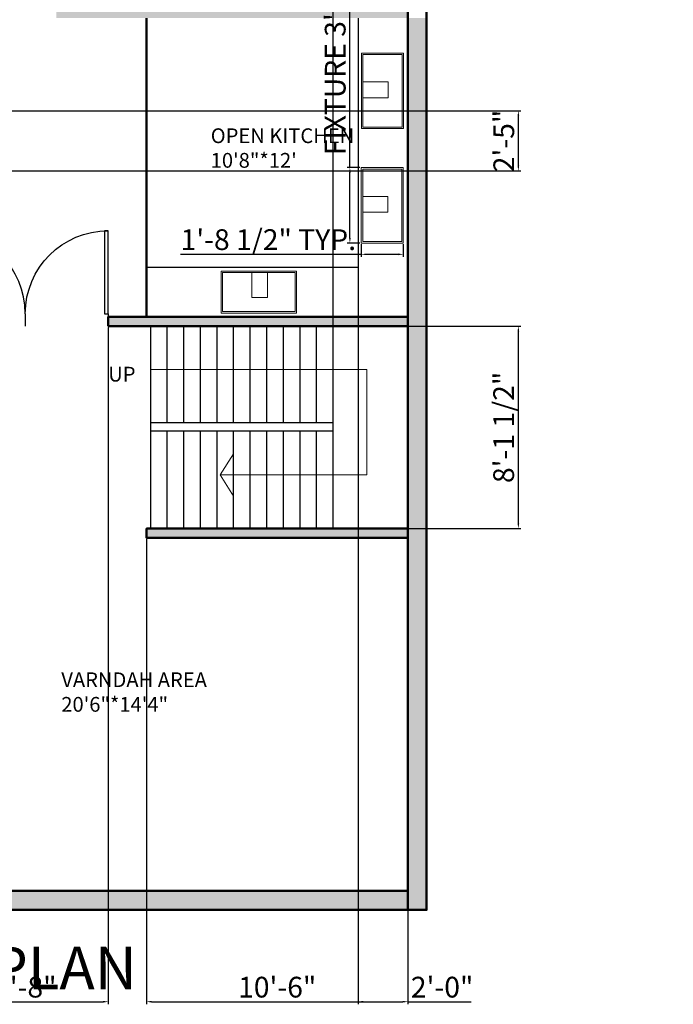
# Model space of a CAD drawing. Units: inches. Extents: x 1477 to 2233, y 1388 to 2326.
# Tile 2 of 4: x 1917 to 2233, y 1396 to 1870. Entities that reach past the tile are written whole.
import ezdxf

# ---------------------------------------------------------------- set-up
doc = ezdxf.new("R2010")
doc.units = ezdxf.units.IN
for name, color, linetype, lineweight in [('A-ANNO-DIMS', 2, 'Continuous', 18), ('A-ANNO-SYMB', 7, 'Continuous', 18), ('A-ANNO-TEXT', 7, 'Continuous', 35), ('A-AREA-IDEN', 7, 'Continuous', 18), ('A-DOOR', 4, 'Continuous', 25), ('A-FLOR-CASE', 9, 'Continuous', 25), ('A-FLOR-FIXT', 8, 'Continuous', 18), ('A-FLOR-STRS', 7, 'Continuous', 25), ('A-WALL-PATT', 10, 'Continuous', 13), ('wall', 10, 'Continuous', 50)]:
    doc.layers.add(name, color=color, linetype=linetype, lineweight=lineweight)
doc.styles.get("Standard").update_dxf_attribs({"font": 'arial.ttf'})
doc.dimstyles.new('ISO-25', dxfattribs={"dimtxt": 10, "dimasz": 2.5, "dimexe": 1.25, "dimexo": 0.625, "dimtad": 1, "dimdec": 0, "dimlunit": 4, "dimtxsty": 'Standard', "dimcen": 2.5, "dimadec": 0, "dimazin": 0, "dimtfac": 1, "dimtdec": 0, "dimtmove": 0, "dimatfit": 3, "dimfxl": 1, "dimarcsym": 0})

# ---------------------------------------------------------------- blocks, each defined once
blk = doc.blocks.new('*U2')
for p, q in [((0, 0), (0, -6)), ((40, 0), (40, -6))]:
    blk.add_line(p, q)
blk.add_lwpolyline([(0, 0), (0, 40), (1.75, 40), (1.75, 0)], close=True)
blk.add_arc((0, 0), 40, 0, 90)
blk = doc.blocks.new('KITCHEN-FIXTURE')
for points in [[(0, 20.26), (36.38, 20.26), (36.38, 0), (0, 0)], [(0.72, 19.54), (35.67, 19.54), (35.67, 0.72), (0.72, 0.72)], [(14.83, 19.54), (22.43, 19.54), (22.43, 7.46), (14.83, 7.46)]]:
    blk.add_lwpolyline(points, close=True)
blk = doc.blocks.new('*D25')
at = {"layer": 'A-ANNO-DIMS', "color": 0, "lineweight": -2, "transparency": 16777216}
for p, q in [((2033, 1898.51), (2033, 1887.14)), ((2104.61, 1898.51), (2104.61, 1887.14)), ((2035.5, 1888.39), (2102.11, 1888.39)), ((2104.61, 1888.39), (2232.55, 1888.39))]:
    blk.add_line(p, q, dxfattribs=at)
at = {"layer": 'A-ANNO-DIMS', "color": 0, "transparency": 16777216}
for points in [[(2035.5, 1888.81), (2035.5, 1887.97), (2033, 1888.39)], [(2102.11, 1888.81), (2102.11, 1887.97), (2104.61, 1888.39)]]:
    blk.add_solid(points, dxfattribs=at)
at = {"layer": 'Defpoints', "color": 0, "transparency": 16777216}
for p in [(2033, 1899.13), (2104.61, 1899.13), (2104.61, 1888.39)]:
    blk.add_point(p, dxfattribs=at)
at = {"layer": 'A-ANNO-DIMS', "color": 0, "transparency": 16777216, "insert": (2169.83, 1894.18), "char_height": 10, "attachment_point": 5}
blk.add_mtext('BED 5\'-11 1/2" TYP.', dxfattribs=at)
blk = doc.blocks.new('*D29')
at = {"layer": 'A-ANNO-DIMS', "color": 0, "lineweight": -2, "transparency": 16777216}
for p, q in [((2076.64, 1799.12), (2076.64, 1950.21)), ((2081.48, 1799.12), (2075.39, 1799.12)), ((2076.64, 1765.24), (2076.64, 1796.62)), ((2081.48, 1762.74), (2075.39, 1762.74))]:
    blk.add_line(p, q, dxfattribs=at)
at = {"layer": 'A-ANNO-DIMS', "color": 0, "transparency": 16777216}
for points in [[(2076.23, 1796.62), (2077.06, 1796.62), (2076.64, 1799.12)], [(2076.23, 1765.24), (2077.06, 1765.24), (2076.64, 1762.74)]]:
    blk.add_solid(points, dxfattribs=at)
at = {"layer": 'Defpoints', "color": 0, "transparency": 16777216}
for p in [(2076.64, 1799.12), (2082.1, 1799.12), (2082.1, 1762.74)]:
    blk.add_point(p, dxfattribs=at)
at = {"layer": 'A-ANNO-DIMS', "color": 0, "transparency": 16777216, "insert": (2070.85, 1875.92), "char_height": 10, "attachment_point": 5, "rotation": 90}
blk.add_mtext('FIXTURE 3\'-0 1/2" TYP.', dxfattribs=at)
blk = doc.blocks.new('*D30')
at = {"layer": 'A-ANNO-DIMS', "color": 0, "lineweight": -2, "transparency": 16777216}
for p, q in [((2082.1, 1762.11), (2082.1, 1756.03)), ((2102.36, 1762.11), (2102.36, 1756.03)), ((2082.1, 1757.28), (1995.04, 1757.28)), ((2099.86, 1757.28), (2084.6, 1757.28))]:
    blk.add_line(p, q, dxfattribs=at)
at = {"layer": 'A-ANNO-DIMS', "color": 0, "transparency": 16777216}
for points in [[(2084.6, 1757.7), (2084.6, 1756.87), (2082.1, 1757.28)], [(2099.86, 1757.7), (2099.86, 1756.87), (2102.36, 1757.28)]]:
    blk.add_solid(points, dxfattribs=at)
at = {"layer": 'Defpoints', "color": 0, "transparency": 16777216}
for p in [(2082.1, 1762.74), (2102.36, 1762.74), (2082.1, 1757.28)]:
    blk.add_point(p, dxfattribs=at)
at = {"layer": 'A-ANNO-DIMS', "color": 0, "transparency": 16777216, "insert": (2037.32, 1763.08), "char_height": 10, "attachment_point": 5}
blk.add_mtext('1\'-8 1/2" TYP.', dxfattribs=at)
blk = doc.blocks.new('*D33')
at = {"layer": 'A-ANNO-DIMS', "color": 0, "lineweight": -2, "transparency": 16777216}
for p, q in [((1880.17, 1722.05), (1880.17, 1395.67)), ((1960.17, 1722.05), (1960.17, 1395.67)), ((1882.67, 1396.92), (1957.67, 1396.92))]:
    blk.add_line(p, q, dxfattribs=at)
at = {"layer": 'A-ANNO-DIMS', "color": 0, "transparency": 16777216}
for points in [[(1882.67, 1397.34), (1882.67, 1396.51), (1880.17, 1396.92)], [(1957.67, 1397.34), (1957.67, 1396.51), (1960.17, 1396.92)]]:
    blk.add_solid(points, dxfattribs=at)
at = {"layer": 'Defpoints', "color": 0, "transparency": 16777216}
for p in [(1880.17, 1722.67), (1960.17, 1722.67), (1960.17, 1396.92)]:
    blk.add_point(p, dxfattribs=at)
at = {"layer": 'A-ANNO-DIMS', "color": 0, "transparency": 16777216, "insert": (1920.17, 1402.65), "char_height": 10, "attachment_point": 5}
blk.add_mtext('6\'-8"', dxfattribs=at)
blk = doc.blocks.new('*D34')
at = {"layer": 'A-ANNO-DIMS', "color": 0, "lineweight": -2, "transparency": 16777216}
for p, q in [((1978.61, 1619.91), (1978.61, 1395.67)), ((2104.61, 1619.91), (2104.61, 1395.67)), ((1981.11, 1396.92), (2102.11, 1396.92))]:
    blk.add_line(p, q, dxfattribs=at)
at = {"layer": 'A-ANNO-DIMS', "color": 0, "transparency": 16777216}
for points in [[(1981.11, 1397.34), (1981.11, 1396.51), (1978.61, 1396.92)], [(2102.11, 1397.34), (2102.11, 1396.51), (2104.61, 1396.92)]]:
    blk.add_solid(points, dxfattribs=at)
at = {"layer": 'Defpoints', "color": 0, "transparency": 16777216}
for p in [(1978.61, 1620.53), (2104.61, 1620.53), (2104.61, 1396.92)]:
    blk.add_point(p, dxfattribs=at)
at = {"layer": 'A-ANNO-DIMS', "color": 0, "transparency": 16777216, "insert": (2041.61, 1402.65), "char_height": 10, "attachment_point": 5}
blk.add_mtext('10\'-6"', dxfattribs=at)
blk = doc.blocks.new('*D35')
at = {"layer": 'A-ANNO-DIMS', "color": 0, "lineweight": -2, "transparency": 16777216}
for p, q in [((2068.61, 1625.95), (2068.61, 2252.67)), ((2071.11, 2251.42), (2102.11, 2251.42)), ((2104.61, 1625.66), (2104.61, 2252.67))]:
    blk.add_line(p, q, dxfattribs=at)
at = {"layer": 'A-ANNO-DIMS', "color": 0, "transparency": 16777216}
for points in [[(2071.11, 2251.84), (2071.11, 2251.01), (2068.61, 2251.42)], [(2102.11, 2251.84), (2102.11, 2251.01), (2104.61, 2251.42)]]:
    blk.add_solid(points, dxfattribs=at)
at = {"layer": 'Defpoints', "color": 0, "transparency": 16777216}
for p in [(2104.61, 2251.42), (2068.61, 1625.33), (2104.61, 1625.03)]:
    blk.add_point(p, dxfattribs=at)
at = {"layer": 'A-ANNO-DIMS', "color": 0, "transparency": 16777216, "insert": (2086.61, 2257.16), "char_height": 10, "attachment_point": 5}
blk.add_mtext('3\'-0"', dxfattribs=at)
blk = doc.blocks.new('*D36')
at = {"layer": 'A-ANNO-DIMS', "color": 0, "lineweight": -2, "transparency": 16777216}
for p, q in [((2105.23, 1722.67), (2159.11, 1722.67)), ((2157.86, 1627.53), (2157.86, 1720.17)), ((2105.23, 1625.03), (2159.11, 1625.03))]:
    blk.add_line(p, q, dxfattribs=at)
at = {"layer": 'A-ANNO-DIMS', "color": 0, "transparency": 16777216}
for points in [[(2157.44, 1720.17), (2158.27, 1720.17), (2157.86, 1722.67)], [(2157.44, 1627.53), (2158.27, 1627.53), (2157.86, 1625.03)]]:
    blk.add_solid(points, dxfattribs=at)
at = {"layer": 'Defpoints', "color": 0, "transparency": 16777216}
for p in [(2104.61, 1722.67), (2157.86, 1722.67), (2104.61, 1625.03)]:
    blk.add_point(p, dxfattribs=at)
at = {"layer": 'A-ANNO-DIMS', "color": 0, "transparency": 16777216, "insert": (2152.06, 1673.85), "char_height": 10, "attachment_point": 5, "rotation": 90}
blk.add_mtext('8\'-1 1/2"', dxfattribs=at)
blk = doc.blocks.new('*D37')
at = {"layer": 'A-ANNO-DIMS', "color": 0, "lineweight": -2, "transparency": 16777216}
for p, q in [((2080.61, 1870.55), (2080.61, 1395.67)), ((2104.61, 1870.55), (2104.61, 1395.67)), ((2083.11, 1396.92), (2102.11, 1396.92)), ((2104.61, 1396.92), (2135.11, 1396.92))]:
    blk.add_line(p, q, dxfattribs=at)
at = {"layer": 'A-ANNO-DIMS', "color": 0, "transparency": 16777216}
for points in [[(2083.11, 1397.34), (2083.11, 1396.51), (2080.61, 1396.92)], [(2102.11, 1397.34), (2102.11, 1396.51), (2104.61, 1396.92)]]:
    blk.add_solid(points, dxfattribs=at)
at = {"layer": 'Defpoints', "color": 0, "transparency": 16777216}
for p in [(2080.61, 1871.17), (2104.61, 1871.17), (2104.61, 1396.92)]:
    blk.add_point(p, dxfattribs=at)
at = {"layer": 'A-ANNO-DIMS', "color": 0, "transparency": 16777216, "insert": (2121.11, 1402.65), "char_height": 10, "attachment_point": 5}
blk.add_mtext('2\'-0"', dxfattribs=at)
blk = doc.blocks.new('*D44')
at = {"layer": 'A-ANNO-DIMS', "color": 0, "lineweight": -2, "transparency": 16777216}
for p, q in [((1855.11, 1826.44), (2159.11, 1826.44)), ((2157.86, 1799.98), (2157.86, 1823.94)), ((1855.35, 1797.48), (2159.11, 1797.48))]:
    blk.add_line(p, q, dxfattribs=at)
at = {"layer": 'A-ANNO-DIMS', "color": 0, "transparency": 16777216}
for points in [[(2157.44, 1823.94), (2158.27, 1823.94), (2157.86, 1826.44)], [(2157.44, 1799.98), (2158.27, 1799.98), (2157.86, 1797.48)]]:
    blk.add_solid(points, dxfattribs=at)
at = {"layer": 'Defpoints', "color": 0, "transparency": 16777216}
for p in [(1854.49, 1826.44), (2157.86, 1826.44), (1854.73, 1797.48)]:
    blk.add_point(p, dxfattribs=at)
at = {"layer": 'A-ANNO-DIMS', "color": 0, "transparency": 16777216, "insert": (2152.13, 1811.96), "char_height": 10, "attachment_point": 5, "rotation": 90}
blk.add_mtext('2\'-5"', dxfattribs=at)

msp = doc.modelspace()

# ---------------------------------------------------------------- hatches: boundary and pattern name
at = {"layer": 'A-WALL-PATT'}
h = msp.add_hatch(color=256, dxfattribs=at)
h.dxf.hatch_style = 1
h.paths.add_polyline_path([(2104.61, 2036.17), (1979.11, 2036.17), (1979.11, 2031.67), (2104.61, 2031.67)])
h.paths.add_polyline_path([(1983.61, 2031.67), (1979.11, 2031.67), (1979.11, 2027.53), (1983.61, 2027.53)])
h.paths.add_polyline_path([(1983.61, 2037.7), (1979.11, 2037.7), (1979.11, 2036.17), (1983.61, 2036.17)])
h.paths.add_polyline_path([(2113.61, 2207.17), (2104.61, 2207.17), (2104.61, 2031.67), (2113.61, 2031.67)])
h.paths.add_polyline_path([(2104.61, 2207.17), (1859.11, 2207.17), (1859.11, 2198.17), (2104.61, 2198.17)])
h.paths.add_polyline_path([(1983.61, 2198.17), (1979.16, 2198.17), (1979.16, 2127.87), (1979.11, 2070.31), (1983.61, 2070.31)])
h.paths.add_polyline_path([(1979.11, 2078.17), (1906.33, 2078.17), (1906.33, 2073.67), (1979.11, 2073.67)])
h.paths.add_polyline_path([(1859.11, 2198.17), (1854.61, 2198.17), (1854.61, 2078.17), (1859.11, 2078.17)])
h.paths.add_polyline_path([(1866.33, 2078.17), (1848.79, 2078.17), (1848.79, 2073.67), (1866.33, 2073.67)])
h.paths.add_polyline_path([(1859.11, 2207.17), (1734.61, 2207.17), (1734.61, 2198.17), (1859.11, 2198.17)])
h.paths.add_polyline_path([(1734.61, 2207.17), (1601.11, 2207.17), (1601.11, 2198.17), (1610.11, 2198.17), (1734.61, 2198.17)])
h.paths.add_polyline_path([(1734.61, 2198.17), (1730.11, 2198.17), (1730.11, 2069.66), (1734.61, 2069.66)])
h.paths.add_polyline_path([(1808.79, 2078.17), (1734.61, 2078.17), (1734.61, 2073.67), (1808.79, 2073.67)])
h.paths.add_polyline_path([(1610.11, 2198.17), (1601.11, 2198.17), (1601.11, 1450.43), (1610.11, 1450.43)])
h.paths.add_polyline_path([(2104.61, 1450.43), (1854.61, 1450.43), (1854.61, 1450.17), (1854.34, 1450.13), (1832.24, 1450.13), (1830.34, 1450.13), (1830.34, 1450.03), (1775.35, 1450.03), (1755.43, 1450.03), (1713.79, 1450.14), (1713.79, 1450.03), (1693.87, 1450.03), (1638.87, 1450.03), (1610.11, 1450.17), (1610.11, 1450.43), (1601.11, 1450.43), (1601.11, 1441.17), (2104.61, 1441.17)])
h.paths.add_polyline_path([(2113.61, 1871.17), (2104.61, 1871.17), (2104.61, 1441.17), (2113.61, 1441.17)])
h.paths.add_polyline_path([(1734.61, 1598.17), (1730.11, 1598.17), (1730.11, 1450.43), (1734.61, 1450.43)])
h = msp.add_hatch(color=256, dxfattribs=at)
h.dxf.hatch_style = 1
h.paths.add_polyline_path([(1734.61, 1993.71), (1730.11, 1993.71), (1730.11, 1875.67), (1734.61, 1875.67)])
h.paths.add_polyline_path([(1730.11, 1875.67), (1610.11, 1875.67), (1610.11, 1871.17), (1730.11, 1871.17)])
h.paths.add_polyline_path([(1776.57, 1875.67), (1730.11, 1875.67), (1730.11, 1871.17), (1776.57, 1871.17)])
h.paths.add_polyline_path([(1896.07, 1875.67), (1815.6, 1875.67), (1815.6, 1871.17), (1896.07, 1871.17)])
h.paths.add_polyline_path([(2104.61, 1875.67), (1935.11, 1875.67), (1935.11, 1871.17), (2104.61, 1871.17)])
h.paths.add_polyline_path([(1734.61, 1871.17), (1730.11, 1871.17), (1730.11, 1727.17), (1734.61, 1727.17)])
h.paths.add_polyline_path([(1775, 1727.17), (1726.93, 1727.17), (1726.93, 1722.67), (1775, 1722.67)])
h.paths.add_polyline_path([(1880.17, 1727.17), (1814.04, 1727.17), (1814.04, 1722.67), (1880.17, 1722.67)])
h.paths.add_polyline_path([(1858.61, 1722.67), (1854.11, 1722.67), (1854.12, 1598.17), (1858.61, 1598.17)])
h.paths.add_polyline_path([(1854.12, 1602.67), (1780.08, 1602.67), (1780.08, 1598.17), (1854.12, 1598.17)])
h.paths.add_polyline_path([(1740.08, 1602.67), (1722.89, 1602.67), (1722.89, 1598.17), (1740.08, 1598.17)])
h.paths.add_polyline_path([(1682.89, 1602.67), (1610.11, 1602.67), (1610.11, 1598.17), (1682.89, 1598.17)])
h.paths.add_polyline_path([(1859.11, 1598.17), (1854.61, 1598.17), (1854.61, 1450.43), (1859.11, 1450.43)])
h.paths.add_polyline_path([(2104.61, 1727.17), (1960.17, 1727.17), (1960.17, 1722.67), (2104.61, 1722.67)])
h.paths.add_polyline_path([(2104.61, 1625.03), (1978.61, 1625.03), (1978.61, 1620.53), (2104.61, 1620.53)])

# ---------------------------------------------------------------- linework, layer by layer
at = {"layer": 'A-ANNO-SYMB'}
for p, q in [((1980.61, 1701.71), (2084.78, 1701.71)), ((2084.78, 1701.71), (2084.78, 1650.9)), ((2014.08, 1650.9), (2020.61, 1661.09)), ((2084.78, 1650.9), (2014.08, 1650.9)), ((2014.08, 1650.9), (2020.61, 1640.72))]:
    msp.add_line(p, q, dxfattribs=at)
at = {"layer": 'A-FLOR-CASE'}
for p, q in [((2080.61, 1871.17), (2080.61, 1751.17)), ((1978.61, 1727.17), (1978.61, 1751.17)), ((1978.61, 1751.17), (2080.61, 1751.17))]:
    msp.add_line(p, q, dxfattribs=at)
at = {"layer": 'A-FLOR-STRS'}
for p, q in [((1980.61, 1625.33), (1980.61, 1722.67)), ((1988.61, 1676), (1988.61, 1722.67)), ((1996.61, 1676), (1996.61, 1722.67)), ((2004.61, 1676), (2004.61, 1722.67)), ((2012.61, 1676), (2012.61, 1722.67)), ((2020.61, 1676), (2020.61, 1722.67)), ((2028.61, 1676), (2028.61, 1722.67)), ((2036.61, 1676), (2036.61, 1722.67)), ((2044.61, 1676), (2044.61, 1722.67)), ((2052.61, 1676), (2052.61, 1722.67)), ((2060.61, 1676), (2060.61, 1722.67)), ((2068.61, 1625.33), (2068.61, 1722.67)), ((2068.61, 1676), (1980.61, 1676)), ((2068.61, 1672), (1980.61, 1672)), ((1988.61, 1625.33), (1988.61, 1672)), ((1996.61, 1625.33), (1996.61, 1672)), ((2004.61, 1625.33), (2004.61, 1672)), ((2012.61, 1625.33), (2012.61, 1672)), ((2020.61, 1625.33), (2020.61, 1672)), ((2028.61, 1625.33), (2028.61, 1672)), ((2036.61, 1625.33), (2036.61, 1672)), ((2044.61, 1625.33), (2044.61, 1672)), ((2052.61, 1625.33), (2052.61, 1672)), ((2060.61, 1625.33), (2060.61, 1672)), ((2068.61, 1625.33), (2056.61, 1625.33)), ((2104.61, 1625.03), (2068.61, 1625.33))]:
    msp.add_line(p, q, dxfattribs=at)
at = {"layer": 'wall'}
for p, q in [((1978.61, 1727.17), (1978.61, 1871.17)), ((2104.61, 1871.17), (2104.61, 1727.17)), ((2113.61, 1871.17), (2113.61, 1722.67)), ((2113.61, 1441.17), (2113.61, 1739.19)), ((2104.61, 1727.17), (2104.61, 1732.5)), ((1960.17, 1727.17), (2034.21, 1727.17)), ((2104.61, 1727.17), (1978.61, 1727.17)), ((1978.61, 1722.67), (1960.17, 1722.67)), ((2104.61, 1722.67), (1978.61, 1722.67)), ((2104.61, 1450.43), (2104.61, 1722.67)), ((1978.61, 1625.03), (2104.61, 1625.03)), ((1978.61, 1625.03), (1978.61, 1620.53)), ((1978.61, 1620.53), (2104.61, 1620.53)), ((1859.11, 1450.43), (2104.61, 1450.43)), ((1859.11, 1441.17), (2113.61, 1441.17))]:
    msp.add_line(p, q, dxfattribs=at)
for points in [[(2104.61, 2207.17), (2113.61, 2207.17), (2113.61, 1441.17), (2104.61, 1441.17)], [(1960.17, 1722.67), (2104.61, 1722.67), (2104.61, 1727.17), (1960.17, 1727.17)], [(2104.61, 1625.03), (1978.61, 1625.03), (1978.61, 1620.53), (2104.61, 1620.53)], [(2104.61, 1450.43), (1601.11, 1450.43), (1601.11, 1441.17), (2104.61, 1441.17)]]:
    msp.add_lwpolyline(points, close=True, dxfattribs=at)

# ---------------------------------------------------------------- block references
at = {"layer": 'A-DOOR'}
msp.add_blockref('*U2', (1880.17, 1728.67), dxfattribs=at)
at = {"layer": 'A-DOOR', "xscale": -1}
msp.add_blockref('*U2', (1960.17, 1728.67), dxfattribs=at)
at = {"layer": 'A-FLOR-FIXT'}
for p, rotation in [((2102.5, 1817.96), 90.00000000000006), ((2102.36, 1762.74), 89.99999999999736)]:
    msp.add_blockref('KITCHEN-FIXTURE', p, dxfattribs=dict(at, rotation=rotation))
msp.add_blockref('KITCHEN-FIXTURE', (2014.54, 1728.96), dxfattribs=at)

# ---------------------------------------------------------------- texts
at = {"layer": 'A-ANNO-SYMB', "insert": (1960.15, 1703.06), "char_height": 7.116, "attachment_point": 1}
msp.add_mtext_dynamic_manual_height_columns('UP', width=109.5726, gutter_width=35.58, heights=[0], dxfattribs=at)
at = {"layer": 'A-ANNO-TEXT', "insert": (1683.6, 1423.44), "char_height": 20.5255, "attachment_point": 1}
msp.add_mtext_dynamic_manual_height_columns('GROUND FLOOR PLAN', width=2854.7469, gutter_width=102.63, heights=[0], dxfattribs=at)
at = {"layer": 'A-AREA-IDEN', "char_height": 7.1161, "attachment_point": 1}
for s, insert in [('OPEN KITCHEN\\P10\'8"*12\'', (2009.56, 1818.03)), ('VARNDAH AREA\\P20\'6"*14\'4"', (1937.54, 1555.72))]:
    msp.add_mtext_dynamic_manual_height_columns(s, width=109.5726, gutter_width=35.58, heights=[0], dxfattribs=dict(at, insert=insert))

# ---------------------------------------------------------------- dimensions: what is measured, and where the dimension line sits
at = {"layer": 'A-ANNO-DIMS'}
for base, p1, p2, picture, middle in [((2104.61, 2251.42), (2068.61, 1625.33), (2104.61, 1625.03), '*D35', (2086.61, 2257.16)), ((2104.61, 1396.92), (2080.61, 1871.17), (2104.61, 1871.17), '*D37', (2121.11, 1402.65)), ((1960.17, 1396.92), (1880.17, 1722.67), (1960.17, 1722.67), '*D33', (1920.17, 1402.65)), ((2104.61, 1396.92), (1978.61, 1620.53), (2104.61, 1620.53), '*D34', (2041.61, 1402.65))]:
    dim = msp.add_linear_dim(base=base, p1=p1, p2=p2, dimstyle='ISO-25', override={"dimdec": 1, "dimlfac": 1, "dimrnd": 0, "dimzin": 1, "dimdsep": 46, "dimlunit": 4, "dimfrac": 2}, dxfattribs=at)
    dim.commit()
    dim.dimension.update_dxf_attribs({"geometry": picture, "text_midpoint": middle})
for base, p1, p2, angle, text, picture, middle in [((2076.64, 1799.12), (2082.1, 1762.74), (2082.1, 1799.12), 90, 'FIXTURE <> TYP.', '*D29', (2070.85, 1875.92)), ((2082.1, 1757.28), (2102.36, 1762.74), (2082.1, 1762.74), 180, '<> TYP.', '*D30', (2037.32, 1763.08))]:
    dim = msp.add_linear_dim(base=base, p1=p1, p2=p2, angle=angle, text=text, dimstyle='ISO-25', override={"dimdec": 1, "dimlfac": 1, "dimrnd": 0, "dimzin": 1, "dimdsep": 46, "dimlunit": 4, "dimfrac": 2}, dxfattribs=at)
    dim.commit()
    dim.dimension.update_dxf_attribs({"geometry": picture, "text_midpoint": middle})
dim = msp.add_linear_dim(base=(2104.61, 1888.39), p1=(2033, 1899.13), p2=(2104.61, 1899.13), text='BED <> TYP.', dimstyle='ISO-25', override={"dimdec": 1, "dimlfac": 1, "dimrnd": 0, "dimzin": 1, "dimdsep": 46, "dimlunit": 4, "dimfrac": 2}, dxfattribs=at)
dim.commit()
dim.dimension.update_dxf_attribs({"geometry": '*D25', "text_midpoint": (2169.83, 1894.18)})
for base, p1, p2, picture, middle in [((2157.86, 1826.44), (1854.73, 1797.48), (1854.49, 1826.44), '*D44', (2152.13, 1811.96)), ((2157.86, 1722.67), (2104.61, 1625.03), (2104.61, 1722.67), '*D36', (2152.06, 1673.85))]:
    dim = msp.add_linear_dim(base=base, p1=p1, p2=p2, angle=90, dimstyle='ISO-25', override={"dimdec": 1, "dimlfac": 1, "dimrnd": 0, "dimzin": 1, "dimdsep": 46, "dimlunit": 4, "dimfrac": 2}, dxfattribs=at)
    dim.commit()
    dim.dimension.update_dxf_attribs({"geometry": picture, "text_midpoint": middle})

doc.saveas('drawing.dxf')
